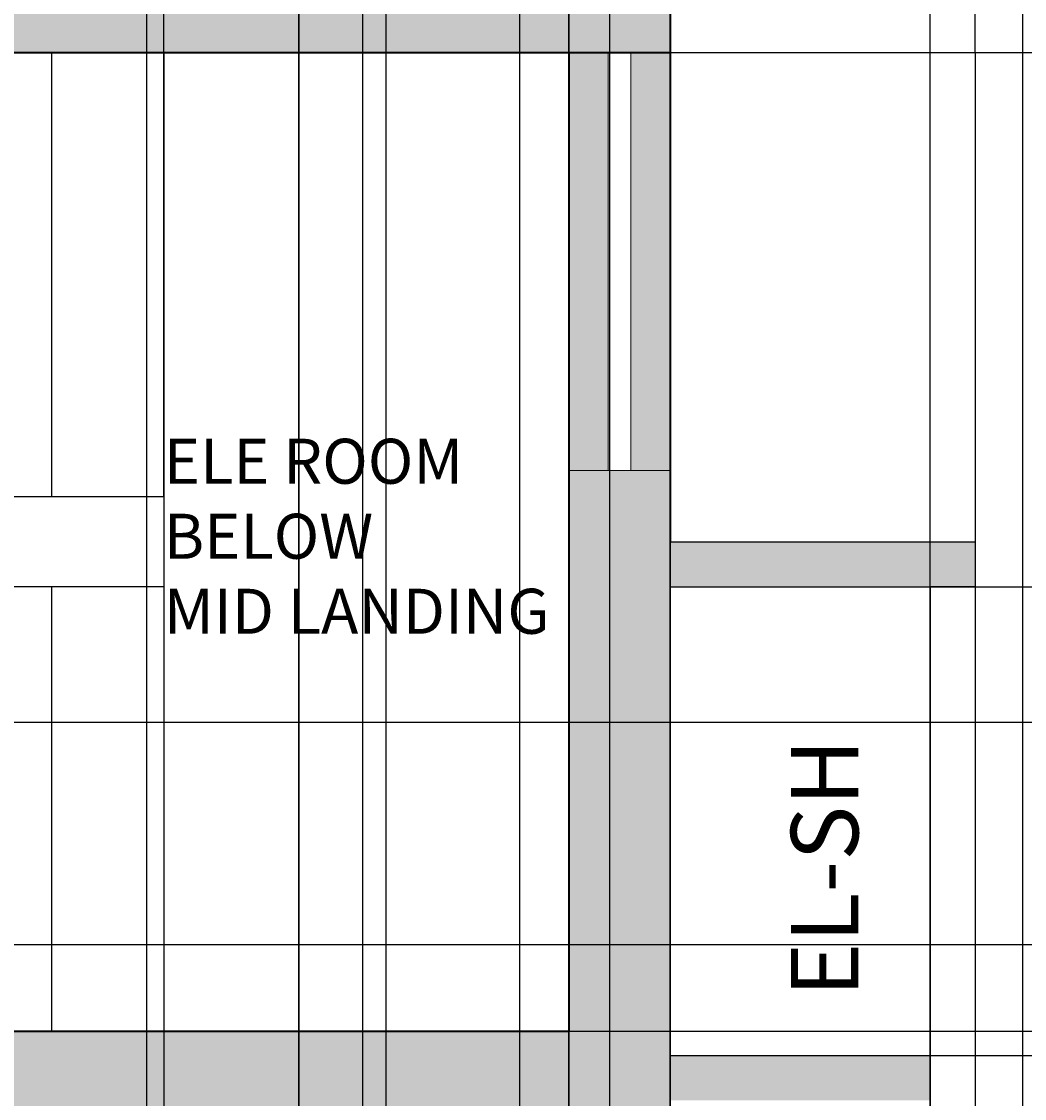
# Model space of a CAD drawing. Units: inches. Extents: x 818 to 1898, y 976 to 2364.
# Tile 49 of 96: x 1657 to 1746, y 1594 to 1690. Entities that reach past the tile are written whole.
import ezdxf

# ---------------------------------------------------------------- set-up
doc = ezdxf.new("R2010")
doc.units = ezdxf.units.IN
doc.header["$LTSCALE"] = 5
doc.header["$MEASUREMENT"] = 0
for name, color, linetype, lineweight in [('A-ANNO-DIMS', 2, 'Continuous', 18), ('A-ANNO-TEXT', 7, 'Continuous', 18), ('A-AREA-IDEN', 7, 'Continuous', 18), ('A-FLOR-SHFT', 7, 'Continuous', 25), ('A-FLOR-STRS', 7, 'Continuous', 25), ('A-GLAZ', 4, 'Continuous', 18), ('A-WALL', 7, 'Continuous', 40)]:
    doc.layers.add(name, color=color, linetype=linetype, lineweight=lineweight)
doc.layers.add('A-GLAZ-PATT', color=141, linetype='Continuous', lineweight=9, true_color=0xadddf7)
doc.layers.add('A-WALL-PATT', color=251, linetype='Continuous', lineweight=13, true_color=0x636466)
doc.styles.get("Standard").update_dxf_attribs({"font": 'arial.ttf'})
doc.dimstyles.get("Standard").update_dxf_attribs({"dimtxt": 0.18, "dimasz": 0.18, "dimexe": 0.18, "dimexo": 0.0625, "dimgap": 0.09, "dimtad": 0, "dimtih": 1, "dimtoh": 1, "dimdec": 4, "dimzin": 0, "dimdsep": 46, "dimtxsty": 'Standard', "dimcen": 0.09, "dimadec": 0, "dimazin": 0, "dimtfac": 1, "dimtdec": 4, "dimtofl": 0, "dimtmove": 0, "dimatfit": 3, "dimfxl": 1, "dimtolj": 1, "dimtzin": 0, "dimarcsym": 0})

# ---------------------------------------------------------------- blocks, each defined once
blk = doc.blocks.new('*D71')
at = {"layer": 'A-ANNO-DIMS', "color": 0, "lineweight": -2, "ltscale": 5, "transparency": 16777216}
for p, q in [((1714.788, 2053.078), (1897.916, 2053.078)), ((1897.736, 2052.898), (1897.736, 1699.76)), ((1897.736, 1346.258), (1897.736, 1699.396)), ((1714.788, 1346.078), (1897.916, 1346.078))]:
    blk.add_line(p, q, dxfattribs=at)
at = {"layer": 'A-ANNO-DIMS', "color": 0, "ltscale": 5, "transparency": 16777216}
for points in [[(1897.706, 2052.898), (1897.766, 2052.898), (1897.736, 2053.078)], [(1897.706, 1346.258), (1897.766, 1346.258), (1897.736, 1346.078)]]:
    blk.add_solid(points, dxfattribs=at)
at = {"layer": 'Defpoints', "color": 0, "ltscale": 5, "transparency": 16777216}
for p in [(1714.725, 2053.078), (1897.736, 2053.078), (1714.725, 1346.078)]:
    blk.add_point(p, dxfattribs=at)
at = {"layer": 'A-ANNO-DIMS', "color": 0, "ltscale": 5, "transparency": 16777216, "insert": (1897.736, 1699.578), "char_height": 0.18, "attachment_point": 5}
blk.add_mtext('\\A1;707', dxfattribs=at)
blk = doc.blocks.new('*D103')
at = {"layer": 'A-ANNO-DIMS', "color": 0, "lineweight": -2, "ltscale": 5, "transparency": 16777216}
for p, q in [((1626.575, 1071.118), (1626.575, 2363.873)), ((1626.755, 2363.693), (1657.699, 2363.693)), ((1689.291, 2363.693), (1658.348, 2363.693)), ((1689.471, 1071.118), (1689.471, 2363.873))]:
    blk.add_line(p, q, dxfattribs=at)
at = {"layer": 'A-ANNO-DIMS', "color": 0, "ltscale": 5, "transparency": 16777216}
for points in [[(1626.755, 2363.723), (1626.755, 2363.663), (1626.575, 2363.693)], [(1689.291, 2363.723), (1689.291, 2363.663), (1689.471, 2363.693)]]:
    blk.add_solid(points, dxfattribs=at)
at = {"layer": 'Defpoints', "color": 0, "ltscale": 5, "transparency": 16777216}
for p in [(1689.471, 2363.693), (1626.575, 1071.055), (1689.471, 1071.055)]:
    blk.add_point(p, dxfattribs=at)
at = {"layer": 'A-ANNO-DIMS', "color": 0, "ltscale": 5, "transparency": 16777216, "insert": (1658.023, 2363.693), "char_height": 0.18, "attachment_point": 5}
blk.add_mtext('\\A1;62.9', dxfattribs=at)
blk = doc.blocks.new('*D104')
at = {"layer": 'A-ANNO-DIMS', "color": 0, "lineweight": -2, "ltscale": 5, "transparency": 16777216}
for p, q in [((1689.471, 1071.118), (1689.471, 2363.873)), ((1689.651, 2363.693), (1717.401, 2363.693)), ((1745.903, 2363.693), (1718.154, 2363.693)), ((1746.083, 1071.118), (1746.083, 2363.873))]:
    blk.add_line(p, q, dxfattribs=at)
at = {"layer": 'A-ANNO-DIMS', "color": 0, "ltscale": 5, "transparency": 16777216}
for points in [[(1689.651, 2363.723), (1689.651, 2363.663), (1689.471, 2363.693)], [(1745.903, 2363.723), (1745.903, 2363.663), (1746.083, 2363.693)]]:
    blk.add_solid(points, dxfattribs=at)
at = {"layer": 'Defpoints', "color": 0, "ltscale": 5, "transparency": 16777216}
for p in [(1746.083, 2363.693), (1689.471, 1071.055), (1746.083, 1071.055)]:
    blk.add_point(p, dxfattribs=at)
at = {"layer": 'A-ANNO-DIMS', "color": 0, "ltscale": 5, "transparency": 16777216, "insert": (1717.777, 2363.693), "char_height": 0.18, "attachment_point": 5}
blk.add_mtext('\\A1;56.61', dxfattribs=at)
blk = doc.blocks.new('*D118')
at = {"layer": 'A-ANNO-DIMS', "color": 0, "lineweight": -2, "ltscale": 5, "transparency": 16777216}
for p, q in [((1766.29, 1627.505), (818.026, 1627.505)), ((818.206, 1627.325), (818.206, 1586.526)), ((818.206, 1545.363), (818.206, 1586.162)), ((1766.29, 1545.183), (818.026, 1545.183))]:
    blk.add_line(p, q, dxfattribs=at)
at = {"layer": 'A-ANNO-DIMS', "color": 0, "ltscale": 5, "transparency": 16777216}
for points in [[(818.176, 1627.325), (818.236, 1627.325), (818.206, 1627.505)], [(818.176, 1545.363), (818.236, 1545.363), (818.206, 1545.183)]]:
    blk.add_solid(points, dxfattribs=at)
at = {"layer": 'Defpoints', "color": 0, "ltscale": 5, "transparency": 16777216}
for p in [(818.206, 1627.505), (1766.352, 1627.505), (1766.352, 1545.183)]:
    blk.add_point(p, dxfattribs=at)
at = {"layer": 'A-ANNO-DIMS', "color": 0, "ltscale": 5, "transparency": 16777216, "insert": (818.206, 1586.344), "char_height": 0.18, "attachment_point": 5}
blk.add_mtext('\\A1;82.32', dxfattribs=at)
blk = doc.blocks.new('*D119')
at = {"layer": 'A-ANNO-DIMS', "color": 0, "lineweight": -2, "ltscale": 5, "transparency": 16777216}
for p, q in [((1766.29, 1716.987), (818.026, 1716.987)), ((818.206, 1716.807), (818.206, 1672.428)), ((818.206, 1627.685), (818.206, 1672.064)), ((1766.29, 1627.505), (818.026, 1627.505))]:
    blk.add_line(p, q, dxfattribs=at)
at = {"layer": 'A-ANNO-DIMS', "color": 0, "ltscale": 5, "transparency": 16777216}
for points in [[(818.176, 1716.807), (818.236, 1716.807), (818.206, 1716.987)], [(818.176, 1627.685), (818.236, 1627.685), (818.206, 1627.505)]]:
    blk.add_solid(points, dxfattribs=at)
at = {"layer": 'Defpoints', "color": 0, "ltscale": 5, "transparency": 16777216}
for p in [(818.206, 1716.987), (1766.352, 1716.987), (1766.352, 1627.505)]:
    blk.add_point(p, dxfattribs=at)
at = {"layer": 'A-ANNO-DIMS', "color": 0, "ltscale": 5, "transparency": 16777216, "insert": (818.206, 1672.246), "char_height": 0.18, "attachment_point": 5}
blk.add_mtext('\\A1;89.48', dxfattribs=at)
blk = doc.blocks.new('*D154')
at = {"layer": 'A-ANNO-DIMS', "color": 0, "lineweight": -2, "ltscale": 5, "transparency": 16777216}
for p, q in [((1701.369, 1290.141), (1701.369, 2363.873)), ((1701.549, 2363.693), (1705.22, 2363.693)), ((1709.189, 2363.693), (1705.518, 2363.693)), ((1709.369, 1298.141), (1709.369, 2363.873))]:
    blk.add_line(p, q, dxfattribs=at)
at = {"layer": 'A-ANNO-DIMS', "color": 0, "ltscale": 5, "transparency": 16777216}
for points in [[(1701.549, 2363.723), (1701.549, 2363.663), (1701.369, 2363.693)], [(1709.189, 2363.723), (1709.189, 2363.663), (1709.369, 2363.693)]]:
    blk.add_solid(points, dxfattribs=at)
at = {"layer": 'Defpoints', "color": 0, "ltscale": 5, "transparency": 16777216}
for p in [(1709.369, 2363.693), (1709.369, 1298.078), (1701.369, 1290.078)]:
    blk.add_point(p, dxfattribs=at)
at = {"layer": 'A-ANNO-DIMS', "color": 0, "ltscale": 5, "transparency": 16777216, "insert": (1705.369, 2363.693), "char_height": 0.18, "attachment_point": 5}
blk.add_mtext('\\A1;8', dxfattribs=at)
blk = doc.blocks.new('*D170')
at = {"layer": 'A-ANNO-DIMS', "color": 0, "lineweight": -2, "ltscale": 5, "transparency": 16777216}
for p, q in [((1430.788, 1600.078), (1897.916, 1600.078)), ((1897.736, 1599.898), (1897.736, 1550.76)), ((1897.736, 1501.258), (1897.736, 1550.396)), ((1430.788, 1501.078), (1897.916, 1501.078))]:
    blk.add_line(p, q, dxfattribs=at)
at = {"layer": 'A-ANNO-DIMS', "color": 0, "ltscale": 5, "transparency": 16777216}
for points in [[(1897.706, 1599.898), (1897.766, 1599.898), (1897.736, 1600.078)], [(1897.706, 1501.258), (1897.766, 1501.258), (1897.736, 1501.078)]]:
    blk.add_solid(points, dxfattribs=at)
at = {"layer": 'Defpoints', "color": 0, "ltscale": 5, "transparency": 16777216}
for p in [(1430.725, 1600.078), (1897.736, 1600.078), (1430.725, 1501.078)]:
    blk.add_point(p, dxfattribs=at)
at = {"layer": 'A-ANNO-DIMS', "color": 0, "ltscale": 5, "transparency": 16777216, "insert": (1897.736, 1550.578), "char_height": 0.18, "attachment_point": 5}
blk.add_mtext('\\A1;99', dxfattribs=at)
blk = doc.blocks.new('*D175')
at = {"layer": 'A-ANNO-DIMS', "color": 0, "lineweight": -2, "ltscale": 5, "transparency": 16777216}
for p, q in [((1559.725, 1647.641), (1559.725, 2363.873)), ((1559.905, 2363.693), (1614.445, 2363.693)), ((1669.545, 2363.693), (1615.005, 2363.693)), ((1669.725, 1647.641), (1669.725, 2363.873))]:
    blk.add_line(p, q, dxfattribs=at)
at = {"layer": 'A-ANNO-DIMS', "color": 0, "ltscale": 5, "transparency": 16777216}
for points in [[(1559.905, 2363.723), (1559.905, 2363.663), (1559.725, 2363.693)], [(1669.545, 2363.723), (1669.545, 2363.663), (1669.725, 2363.693)]]:
    blk.add_solid(points, dxfattribs=at)
at = {"layer": 'Defpoints', "color": 0, "ltscale": 5, "transparency": 16777216}
for p in [(1669.725, 2363.693), (1559.725, 1647.578), (1669.725, 1647.578)]:
    blk.add_point(p, dxfattribs=at)
at = {"layer": 'A-ANNO-DIMS', "color": 0, "ltscale": 5, "transparency": 16777216, "insert": (1614.725, 2363.693), "char_height": 0.18, "attachment_point": 5}
blk.add_mtext('\\A1;110', dxfattribs=at)
blk = doc.blocks.new('*D178')
at = {"layer": 'A-ANNO-DIMS', "color": 0, "lineweight": -2, "ltscale": 5, "transparency": 16777216}
for p, q in [((1669.725, 1600.016), (1669.725, 975.663)), ((1705.725, 1600.016), (1705.725, 975.663)), ((1669.905, 975.843), (1687.506, 975.843)), ((1705.545, 975.843), (1687.944, 975.843))]:
    blk.add_line(p, q, dxfattribs=at)
at = {"layer": 'A-ANNO-DIMS', "color": 0, "ltscale": 5, "transparency": 16777216}
for points in [[(1669.905, 975.873), (1669.905, 975.813), (1669.725, 975.843)], [(1705.545, 975.873), (1705.545, 975.813), (1705.725, 975.843)]]:
    blk.add_solid(points, dxfattribs=at)
at = {"layer": 'Defpoints', "color": 0, "ltscale": 5, "transparency": 16777216}
for p in [(1669.725, 1600.078), (1705.725, 1600.078), (1705.725, 975.843)]:
    blk.add_point(p, dxfattribs=at)
at = {"layer": 'A-ANNO-DIMS', "color": 0, "ltscale": 5, "transparency": 16777216, "insert": (1687.725, 975.843), "char_height": 0.18, "attachment_point": 5}
blk.add_mtext('\\A1;36', dxfattribs=at)
blk = doc.blocks.new('*D179')
at = {"layer": 'A-ANNO-DIMS', "color": 0, "lineweight": -2, "ltscale": 5, "transparency": 16777216}
for p, q in [((1669.788, 1687.078), (1897.916, 1687.078)), ((1897.736, 1686.898), (1897.736, 1643.76)), ((1897.736, 1600.258), (1897.736, 1643.396)), ((1669.788, 1600.078), (1897.916, 1600.078))]:
    blk.add_line(p, q, dxfattribs=at)
at = {"layer": 'A-ANNO-DIMS', "color": 0, "ltscale": 5, "transparency": 16777216}
for points in [[(1897.706, 1686.898), (1897.766, 1686.898), (1897.736, 1687.078)], [(1897.706, 1600.258), (1897.766, 1600.258), (1897.736, 1600.078)]]:
    blk.add_solid(points, dxfattribs=at)
at = {"layer": 'Defpoints', "color": 0, "ltscale": 5, "transparency": 16777216}
for p in [(1669.725, 1687.078), (1897.736, 1687.078), (1669.725, 1600.078)]:
    blk.add_point(p, dxfattribs=at)
at = {"layer": 'A-ANNO-DIMS', "color": 0, "ltscale": 5, "transparency": 16777216, "insert": (1897.736, 1643.578), "char_height": 0.18, "attachment_point": 5}
blk.add_mtext('\\A1;87', dxfattribs=at)
blk = doc.blocks.new('*D180')
at = {"layer": 'A-ANNO-DIMS', "color": 0, "lineweight": -2, "ltscale": 5, "transparency": 16777216}
for p, q in [((1599.725, 1639.516), (1599.725, 975.663)), ((1669.725, 1639.516), (1669.725, 975.663)), ((1599.905, 975.843), (1634.507, 975.843)), ((1669.545, 975.843), (1634.943, 975.843))]:
    blk.add_line(p, q, dxfattribs=at)
at = {"layer": 'A-ANNO-DIMS', "color": 0, "ltscale": 5, "transparency": 16777216}
for points in [[(1599.905, 975.873), (1599.905, 975.813), (1599.725, 975.843)], [(1669.545, 975.873), (1669.545, 975.813), (1669.725, 975.843)]]:
    blk.add_solid(points, dxfattribs=at)
at = {"layer": 'Defpoints', "color": 0, "ltscale": 5, "transparency": 16777216}
for p in [(1599.725, 1639.578), (1669.725, 1639.578), (1669.725, 975.843)]:
    blk.add_point(p, dxfattribs=at)
at = {"layer": 'A-ANNO-DIMS', "color": 0, "ltscale": 5, "transparency": 16777216, "insert": (1634.725, 975.843), "char_height": 0.18, "attachment_point": 5}
blk.add_mtext('\\A1;70', dxfattribs=at)
blk = doc.blocks.new('*D185')
at = {"layer": 'A-ANNO-DIMS', "color": 0, "lineweight": -2, "ltscale": 5, "transparency": 16777216}
for p, q in [((1737.903, 1639.578), (1897.916, 1639.578)), ((1897.736, 1639.398), (1897.736, 1618.93)), ((1897.736, 1598.098), (1897.736, 1618.566)), ((1737.903, 1597.918), (1897.916, 1597.918))]:
    blk.add_line(p, q, dxfattribs=at)
at = {"layer": 'A-ANNO-DIMS', "color": 0, "ltscale": 5, "transparency": 16777216}
for points in [[(1897.706, 1639.398), (1897.766, 1639.398), (1897.736, 1639.578)], [(1897.706, 1598.098), (1897.766, 1598.098), (1897.736, 1597.918)]]:
    blk.add_solid(points, dxfattribs=at)
at = {"layer": 'Defpoints', "color": 0, "ltscale": 5, "transparency": 16777216}
for p in [(1737.841, 1639.578), (1897.736, 1639.578), (1737.841, 1597.918)]:
    blk.add_point(p, dxfattribs=at)
at = {"layer": 'A-ANNO-DIMS', "color": 0, "ltscale": 5, "transparency": 16777216, "insert": (1897.736, 1618.748), "char_height": 0.18, "attachment_point": 5}
blk.add_mtext('\\A1;41.66', dxfattribs=at)
blk = doc.blocks.new('*D186')
at = {"layer": 'A-ANNO-DIMS', "color": 0, "lineweight": -2, "ltscale": 5, "transparency": 16777216}
for p, q in [((1714.725, 1549.141), (1714.725, 2363.873)), ((1714.905, 2363.693), (1725.818, 2363.693)), ((1737.661, 2363.693), (1726.748, 2363.693)), ((1737.841, 1549.141), (1737.841, 2363.873))]:
    blk.add_line(p, q, dxfattribs=at)
at = {"layer": 'A-ANNO-DIMS', "color": 0, "ltscale": 5, "transparency": 16777216}
for points in [[(1714.905, 2363.723), (1714.905, 2363.663), (1714.725, 2363.693)], [(1737.661, 2363.723), (1737.661, 2363.663), (1737.841, 2363.693)]]:
    blk.add_solid(points, dxfattribs=at)
at = {"layer": 'Defpoints', "color": 0, "ltscale": 5, "transparency": 16777216}
for p in [(1737.841, 2363.693), (1714.725, 1549.078), (1737.841, 1549.078)]:
    blk.add_point(p, dxfattribs=at)
at = {"layer": 'A-ANNO-DIMS', "color": 0, "ltscale": 5, "transparency": 16777216, "insert": (1726.283, 2363.693), "char_height": 0.18, "attachment_point": 5}
blk.add_mtext('\\A1;23.116', dxfattribs=at)
blk = doc.blocks.new('*D195')
at = {"layer": 'A-ANNO-DIMS', "color": 0, "lineweight": -2, "ltscale": 5, "transparency": 16777216}
for p, q in [((1681.725, 1379.141), (1681.725, 2363.873)), ((1681.905, 2363.693), (1693.505, 2363.693)), ((1705.545, 2363.693), (1693.945, 2363.693)), ((1705.725, 1355.141), (1705.725, 2363.873))]:
    blk.add_line(p, q, dxfattribs=at)
at = {"layer": 'A-ANNO-DIMS', "color": 0, "ltscale": 5, "transparency": 16777216}
for points in [[(1681.905, 2363.723), (1681.905, 2363.663), (1681.725, 2363.693)], [(1705.545, 2363.723), (1705.545, 2363.663), (1705.725, 2363.693)]]:
    blk.add_solid(points, dxfattribs=at)
at = {"layer": 'Defpoints', "color": 0, "ltscale": 5, "transparency": 16777216}
for p in [(1705.725, 2363.693), (1681.725, 1379.078), (1705.725, 1355.078)]:
    blk.add_point(p, dxfattribs=at)
at = {"layer": 'A-ANNO-DIMS', "color": 0, "ltscale": 5, "transparency": 16777216, "insert": (1693.725, 2363.693), "char_height": 0.18, "attachment_point": 5}
blk.add_mtext('\\A1;24', dxfattribs=at)
blk = doc.blocks.new('*D199')
at = {"layer": 'A-ANNO-DIMS', "color": 0, "lineweight": -2, "ltscale": 5, "transparency": 16777216}
for p, q in [((1559.788, 1687.078), (1897.916, 1687.078)), ((1897.736, 1686.898), (1897.736, 1513.154)), ((1897.736, 1339.045), (1897.736, 1512.79)), ((1660.377, 1338.865), (1897.916, 1338.865))]:
    blk.add_line(p, q, dxfattribs=at)
at = {"layer": 'A-ANNO-DIMS', "color": 0, "ltscale": 5, "transparency": 16777216}
for points in [[(1897.706, 1686.898), (1897.766, 1686.898), (1897.736, 1687.078)], [(1897.706, 1339.045), (1897.766, 1339.045), (1897.736, 1338.865)]]:
    blk.add_solid(points, dxfattribs=at)
at = {"layer": 'Defpoints', "color": 0, "ltscale": 5, "transparency": 16777216}
for p in [(1559.725, 1687.078), (1897.736, 1687.078), (1660.314, 1338.865)]:
    blk.add_point(p, dxfattribs=at)
at = {"layer": 'A-ANNO-DIMS', "color": 0, "ltscale": 5, "transparency": 16777216, "insert": (1897.736, 1512.972), "char_height": 0.18, "attachment_point": 5}
blk.add_mtext('\\A1;348.2', dxfattribs=at)
blk = doc.blocks.new('*D212')
at = {"layer": 'A-ANNO-DIMS', "color": 0, "lineweight": -2, "ltscale": 5, "transparency": 16777216}
for p, q in [((1681.725, 1900.016), (1681.725, 975.663)), ((1705.725, 1876.016), (1705.725, 975.663)), ((1681.905, 975.843), (1693.505, 975.843)), ((1705.545, 975.843), (1693.945, 975.843))]:
    blk.add_line(p, q, dxfattribs=at)
at = {"layer": 'A-ANNO-DIMS', "color": 0, "ltscale": 5, "transparency": 16777216}
for points in [[(1681.905, 975.873), (1681.905, 975.813), (1681.725, 975.843)], [(1705.545, 975.873), (1705.545, 975.813), (1705.725, 975.843)]]:
    blk.add_solid(points, dxfattribs=at)
at = {"layer": 'Defpoints', "color": 0, "ltscale": 5, "transparency": 16777216}
for p in [(1681.725, 1900.078), (1705.725, 1876.078), (1705.725, 975.843)]:
    blk.add_point(p, dxfattribs=at)
at = {"layer": 'A-ANNO-DIMS', "color": 0, "ltscale": 5, "transparency": 16777216, "insert": (1693.725, 975.843), "char_height": 0.18, "attachment_point": 5}
blk.add_mtext('\\A1;24', dxfattribs=at)
blk = doc.blocks.new('*D214')
at = {"layer": 'A-ANNO-DIMS', "color": 0, "lineweight": -2, "ltscale": 5, "transparency": 16777216}
for p, q in [((1511.725, 1687.016), (1511.725, 975.663)), ((1714.725, 1687.016), (1714.725, 975.663)), ((1511.905, 975.843), (1612.935, 975.843)), ((1714.545, 975.843), (1613.516, 975.843))]:
    blk.add_line(p, q, dxfattribs=at)
at = {"layer": 'A-ANNO-DIMS', "color": 0, "ltscale": 5, "transparency": 16777216}
for points in [[(1511.905, 975.873), (1511.905, 975.813), (1511.725, 975.843)], [(1714.545, 975.873), (1714.545, 975.813), (1714.725, 975.843)]]:
    blk.add_solid(points, dxfattribs=at)
at = {"layer": 'Defpoints', "color": 0, "ltscale": 5, "transparency": 16777216}
for p in [(1511.725, 1687.078), (1714.725, 1687.078), (1714.725, 975.843)]:
    blk.add_point(p, dxfattribs=at)
at = {"layer": 'A-ANNO-DIMS', "color": 0, "ltscale": 5, "transparency": 16777216, "insert": (1613.225, 975.843), "char_height": 0.18, "attachment_point": 5}
blk.add_mtext('\\A1;203', dxfattribs=at)
blk = doc.blocks.new('*D221')
at = {"layer": 'A-ANNO-DIMS', "color": 0, "lineweight": -2, "ltscale": 5, "transparency": 16777216}
for p, q in [((1668.184, 1696.016), (1668.184, 975.663)), ((1705.725, 1696.016), (1705.725, 975.663)), ((1668.364, 975.843), (1686.561, 975.843)), ((1705.545, 975.843), (1687.348, 975.843))]:
    blk.add_line(p, q, dxfattribs=at)
at = {"layer": 'A-ANNO-DIMS', "color": 0, "ltscale": 5, "transparency": 16777216}
for points in [[(1668.364, 975.873), (1668.364, 975.813), (1668.184, 975.843)], [(1705.545, 975.873), (1705.545, 975.813), (1705.725, 975.843)]]:
    blk.add_solid(points, dxfattribs=at)
at = {"layer": 'Defpoints', "color": 0, "ltscale": 5, "transparency": 16777216}
for p in [(1668.184, 1696.078), (1705.725, 1696.078), (1705.725, 975.843)]:
    blk.add_point(p, dxfattribs=at)
at = {"layer": 'A-ANNO-DIMS', "color": 0, "ltscale": 5, "transparency": 16777216, "insert": (1686.955, 975.843), "char_height": 0.18, "attachment_point": 5}
blk.add_mtext('\\A1;37.54', dxfattribs=at)
blk = doc.blocks.new('*D228')
at = {"layer": 'A-ANNO-DIMS', "color": 0, "lineweight": -2, "ltscale": 5, "transparency": 16777216}
for p, q in [((1687.394, 1802.016), (1687.394, 975.663)), ((1705.725, 1802.016), (1705.725, 975.663)), ((1687.574, 975.843), (1696.174, 975.843)), ((1705.545, 975.843), (1696.945, 975.843))]:
    blk.add_line(p, q, dxfattribs=at)
at = {"layer": 'A-ANNO-DIMS', "color": 0, "ltscale": 5, "transparency": 16777216}
for points in [[(1687.574, 975.873), (1687.574, 975.813), (1687.394, 975.843)], [(1705.545, 975.873), (1705.545, 975.813), (1705.725, 975.843)]]:
    blk.add_solid(points, dxfattribs=at)
at = {"layer": 'Defpoints', "color": 0, "ltscale": 5, "transparency": 16777216}
for p in [(1687.394, 1802.078), (1705.725, 1802.078), (1705.725, 975.843)]:
    blk.add_point(p, dxfattribs=at)
at = {"layer": 'A-ANNO-DIMS', "color": 0, "ltscale": 5, "transparency": 16777216, "insert": (1696.56, 975.843), "char_height": 0.18, "attachment_point": 5}
blk.add_mtext('\\A1;18.33', dxfattribs=at)
blk = doc.blocks.new('*D267')
at = {"layer": 'A-ANNO-DIMS', "color": 0, "lineweight": -2, "ltscale": 5, "transparency": 16777216}
for p, q in [((1714.725, 1687.016), (1714.725, 975.663)), ((1741.841, 1687.016), (1741.841, 975.663)), ((1714.905, 975.843), (1727.818, 975.843)), ((1741.661, 975.843), (1728.748, 975.843))]:
    blk.add_line(p, q, dxfattribs=at)
at = {"layer": 'A-ANNO-DIMS', "color": 0, "ltscale": 5, "transparency": 16777216}
for points in [[(1714.905, 975.873), (1714.905, 975.813), (1714.725, 975.843)], [(1741.661, 975.873), (1741.661, 975.813), (1741.841, 975.843)]]:
    blk.add_solid(points, dxfattribs=at)
at = {"layer": 'Defpoints', "color": 0, "ltscale": 5, "transparency": 16777216}
for p in [(1714.725, 1687.078), (1741.841, 1687.078), (1741.841, 975.843)]:
    blk.add_point(p, dxfattribs=at)
at = {"layer": 'A-ANNO-DIMS', "color": 0, "ltscale": 5, "transparency": 16777216, "insert": (1728.283, 975.843), "char_height": 0.18, "attachment_point": 5}
blk.add_mtext('\\A1;27.116', dxfattribs=at)
blk = doc.blocks.new('*D268')
at = {"layer": 'A-ANNO-DIMS', "color": 0, "lineweight": -2, "ltscale": 5, "transparency": 16777216}
for p, q in [((1741.903, 1890.29), (1897.916, 1890.29)), ((1897.736, 1890.11), (1897.736, 1788.866)), ((1897.736, 1687.258), (1897.736, 1788.502)), ((1741.903, 1687.078), (1897.916, 1687.078))]:
    blk.add_line(p, q, dxfattribs=at)
at = {"layer": 'A-ANNO-DIMS', "color": 0, "ltscale": 5, "transparency": 16777216}
for points in [[(1897.706, 1890.11), (1897.766, 1890.11), (1897.736, 1890.29)], [(1897.706, 1687.258), (1897.766, 1687.258), (1897.736, 1687.078)]]:
    blk.add_solid(points, dxfattribs=at)
at = {"layer": 'Defpoints', "color": 0, "ltscale": 5, "transparency": 16777216}
for p in [(1741.841, 1890.29), (1897.736, 1890.29), (1741.841, 1687.078)]:
    blk.add_point(p, dxfattribs=at)
at = {"layer": 'A-ANNO-DIMS', "color": 0, "ltscale": 5, "transparency": 16777216, "insert": (1897.736, 1788.684), "char_height": 0.18, "attachment_point": 5}
blk.add_mtext('\\A1;203.2', dxfattribs=at)
blk = doc.blocks.new('*D282')
at = {"layer": 'A-ANNO-DIMS', "color": 0, "lineweight": -2, "ltscale": 5, "transparency": 16777216}
for p, q in [((1422.083, 2081.188), (1897.916, 2081.188)), ((1897.736, 2081.008), (1897.736, 1884.315)), ((1897.736, 1687.258), (1897.736, 1883.951)), ((1463.788, 1687.078), (1897.916, 1687.078))]:
    blk.add_line(p, q, dxfattribs=at)
at = {"layer": 'A-ANNO-DIMS', "color": 0, "ltscale": 5, "transparency": 16777216}
for points in [[(1897.706, 2081.008), (1897.766, 2081.008), (1897.736, 2081.188)], [(1897.706, 1687.258), (1897.766, 1687.258), (1897.736, 1687.078)]]:
    blk.add_solid(points, dxfattribs=at)
at = {"layer": 'Defpoints', "color": 0, "ltscale": 5, "transparency": 16777216}
for p in [(1422.02, 2081.188), (1897.736, 2081.188), (1463.725, 1687.078)]:
    blk.add_point(p, dxfattribs=at)
at = {"layer": 'A-ANNO-DIMS', "color": 0, "ltscale": 5, "transparency": 16777216, "insert": (1897.736, 1884.133), "char_height": 0.18, "attachment_point": 5}
blk.add_mtext('\\A1;394.1', dxfattribs=at)
blk = doc.blocks.new('*D291')
at = {"layer": 'A-ANNO-DIMS', "color": 0, "lineweight": -2, "ltscale": 5, "transparency": 16777216}
for p, q in [((1206.788, 1687.078), (1897.916, 1687.078)), ((1897.736, 1686.898), (1897.736, 1647.606)), ((1897.736, 1607.951), (1897.736, 1647.242)), ((1318.956, 1607.771), (1897.916, 1607.771))]:
    blk.add_line(p, q, dxfattribs=at)
at = {"layer": 'A-ANNO-DIMS', "color": 0, "ltscale": 5, "transparency": 16777216}
for points in [[(1897.706, 1686.898), (1897.766, 1686.898), (1897.736, 1687.078)], [(1897.706, 1607.951), (1897.766, 1607.951), (1897.736, 1607.771)]]:
    blk.add_solid(points, dxfattribs=at)
at = {"layer": 'Defpoints', "color": 0, "ltscale": 5, "transparency": 16777216}
for p in [(1206.725, 1687.078), (1897.736, 1687.078), (1318.893, 1607.771)]:
    blk.add_point(p, dxfattribs=at)
at = {"layer": 'A-ANNO-DIMS', "color": 0, "ltscale": 5, "transparency": 16777216, "insert": (1897.736, 1647.424), "char_height": 0.18, "attachment_point": 5}
blk.add_mtext('\\A1;79.3', dxfattribs=at)

msp = doc.modelspace()

# ---------------------------------------------------------------- hatches: boundary and pattern name
at = {"layer": 'A-GLAZ-PATT', "ltscale": 5}
h = msp.add_hatch(color=256, dxfattribs=at)
h.dxf.hatch_style = 1
h.paths.add_polyline_path([(1283.8183, 1504.5782), (1206.7251, 1504.5782), (1206.7251, 1501.0782), (1283.8183, 1501.0782)])
h.paths.add_polyline_path([(1283.8183, 1510.0782), (1206.7251, 1510.0782), (1206.7251, 1506.5782), (1283.8183, 1506.5782)])
h.paths.add_polyline_path([(1490.9163, 1355.0782), (1439.7252, 1355.0782), (1439.7252, 1409.0522), (1436.2252, 1409.0522), (1436.2252, 1351.5782), (1490.9163, 1351.5782)])
h.paths.add_polyline_path([(1434.2252, 1409.0522), (1430.7251, 1409.0522), (1430.7251, 1346.0782), (1435.0799, 1346.0782), (1435.0731, 1346.1152), (1435.1501, 1346.0782), (1490.9163, 1346.0782), (1490.9163, 1349.5782), (1434.2252, 1349.5782)])
h.paths.add_polyline_path([(1714.7251, 1545.0782), (1711.2252, 1545.0782), (1711.2252, 1521.0782), (1714.7251, 1521.0782)])
h.paths.add_polyline_path([(1709.2252, 1545.0782), (1705.7251, 1545.0782), (1705.7251, 1521.0782), (1709.2252, 1521.0782)])
h.paths.add_polyline_path([(1714.7251, 1687.0782), (1711.2252, 1687.0782), (1711.2252, 1649.9029), (1714.7251, 1649.9029)])
h.paths.add_polyline_path([(1709.2252, 1687.0782), (1705.7251, 1687.0782), (1705.7251, 1649.9029), (1709.2252, 1649.9029)])
h.paths.add_polyline_path([(1709.2252, 1745.5584), (1705.7251, 1745.5584), (1705.7251, 1717.3178), (1709.2252, 1717.3178)])
h.paths.add_polyline_path([(1714.7251, 1745.5584), (1711.2252, 1745.5584), (1711.2252, 1717.3178), (1714.7251, 1717.3178)])
h.paths.add_polyline_path([(1714.7251, 2014.5114), (1711.2252, 2014.5114), (1711.2252, 1962.0338), (1714.7251, 1962.0338)])
h.paths.add_polyline_path([(1709.2252, 2014.5114), (1705.7251, 2014.5114), (1705.7251, 1962.0338), (1709.2252, 1962.0338)])
h.paths.add_polyline_path([(1538.5155, 2047.5782), (1485.1216, 2047.5782), (1485.1216, 2044.0782), (1538.5155, 2044.0782)])
h.paths.add_polyline_path([(1538.5155, 2053.0782), (1485.1216, 2053.0782), (1485.1216, 2049.5782), (1538.5155, 2049.5782)])
h.paths.add_polyline_path([(1388.0315, 2047.5782), (1330.305, 2047.5782), (1330.305, 2044.0782), (1388.0315, 2044.0782)])
h.paths.add_polyline_path([(1388.0315, 2053.0782), (1330.305, 2053.0782), (1330.305, 2049.5782), (1388.0315, 2049.5782)])
h.paths.add_polyline_path([(1262.2252, 2019.2871), (1258.7252, 2019.2871), (1258.7252, 1928.9218), (1262.2252, 1928.9218)])
h.paths.add_polyline_path([(1267.7252, 2019.2871), (1264.2252, 2019.2871), (1264.2252, 1928.9218), (1267.7252, 1928.9218)])
h.paths.add_polyline_path([(1262.2252, 1862.9652), (1258.7252, 1862.9652), (1258.7252, 1814.9652), (1262.2252, 1814.9652)])
h.paths.add_polyline_path([(1267.7252, 1862.9652), (1264.2252, 1862.9652), (1264.2252, 1814.9652), (1267.7252, 1814.9652)])
h.paths.add_polyline_path([(1262.2252, 1755.3321), (1258.7252, 1755.3321), (1258.7252, 1707.3321), (1262.2252, 1707.3321)])
h.paths.add_polyline_path([(1267.7252, 1755.3321), (1264.2252, 1755.3321), (1264.2252, 1707.3321), (1267.7252, 1707.3321)])
h.paths.add_polyline_path([(1251.9333, 1692.5782), (1206.7251, 1692.5782), (1206.7251, 1687.0782), (1251.9333, 1687.0782)])
h.paths.add_polyline_path([(1251.9333, 1700.0782), (1206.7251, 1700.0782), (1206.7251, 1694.5782), (1251.9333, 1694.5782)])
at = {"layer": 'A-WALL-PATT', "ltscale": 5}
h = msp.add_hatch(color=256, dxfattribs=at)
h.dxf.hatch_style = 1
h.paths.add_polyline_path([(1267.7252, 1928.9218), (1258.7252, 1928.9218), (1258.7252, 1913.6401), (1250.3029, 1913.6401), (1250.3029, 1878.3919), (1258.7252, 1878.3919), (1258.7252, 1862.9652), (1267.7252, 1862.9652)])
h.paths.add_polyline_path([(1267.7252, 1814.9652), (1258.7252, 1814.9652), (1258.7252, 1755.3321), (1267.7252, 1755.3321)])
h.paths.add_polyline_path([(1463.7251, 1696.0782), (1267.7252, 1696.0782), (1267.7252, 1707.3321), (1258.7252, 1707.3321), (1258.7252, 1700.0782), (1251.9333, 1700.0782), (1251.9333, 1687.0782), (1463.7251, 1687.0782)])
h.paths.add_polyline_path([(1714.7251, 1717.3178), (1705.7251, 1717.3178), (1705.7251, 1696.0782), (1599.7251, 1696.0782), (1599.7251, 1790.0782), (1705.7251, 1790.0782), (1705.7251, 1785.6125), (1714.7251, 1785.6125), (1714.7251, 1827.2125), (1705.7251, 1827.2125), (1705.7251, 1802.0782), (1599.7251, 1802.0782), (1599.7251, 1867.0782), (1705.7251, 1867.0782), (1705.7251, 1857.2125), (1714.7251, 1857.2125), (1714.7251, 1930.0316), (1741.8409, 1930.0316), (1741.8409, 1935.0316), (1714.7251, 1935.0316), (1714.7251, 1957.0338), (1741.8409, 1957.0338), (1741.8409, 1962.0338), (1714.7251, 1962.0338), (1705.7251, 1962.0338), (1705.7251, 1948.0782), (1599.7251, 1948.0782), (1599.7251, 1981.0782), (1590.7252, 1981.0782), (1590.7252, 1941.0782), (1620.7252, 1941.0782), (1705.7251, 1941.0782), (1705.7251, 1876.0782), (1599.7251, 1876.0782), (1599.7251, 1911.0782), (1590.7252, 1911.0782), (1590.7252, 1876.0782), (1429.2252, 1876.0782), (1429.2252, 1867.0782), (1511.7251, 1867.0782), (1528.593, 1867.0782), (1595.7252, 1867.0782), (1595.7252, 1773.0782), (1520.7252, 1773.0782), (1520.7252, 1837.5823), (1532.593, 1837.5823), (1532.593, 1867.0782), (1528.593, 1867.0782), (1528.593, 1841.5823), (1511.7251, 1841.5823), (1511.7251, 1744.9714), (1520.7252, 1744.9714), (1520.7252, 1761.0782), (1595.7252, 1761.0782), (1595.7252, 1696.0782), (1520.7252, 1696.0782), (1520.7252, 1716.0454), (1511.7251, 1716.0454), (1511.7251, 1696.0782), (1511.7251, 1687.0782), (1714.7251, 1687.0782)])
h.paths.add_polyline_path([(1714.7251, 2053.0782), (1714.7251, 2081.1881), (1709.7252, 2081.1881), (1709.7252, 2053.0782), (1681.6446, 2053.0782), (1681.6446, 2081.1881), (1676.6446, 2081.1881), (1676.6446, 2053.0782), (1538.5155, 2053.0782), (1538.5155, 2044.0782), (1590.7252, 2044.0782), (1590.7252, 2011.0782), (1599.7251, 2011.0782), (1599.7251, 2044.0782), (1705.7251, 2044.0782), (1705.7251, 2014.5114), (1714.7251, 2014.5114)])
h.paths.add_polyline_path([(1485.1216, 2053.0782), (1422.02, 2053.0782), (1422.02, 2081.1881), (1413.02, 2081.1881), (1413.02, 2053.0782), (1399.6356, 2053.0782), (1399.6356, 2081.1881), (1390.6356, 2081.1881), (1390.6356, 2053.0782), (1388.0315, 2053.0782), (1388.0315, 2044.0782), (1416.2743, 2044.0782), (1485.1216, 2044.0782)])
h.paths.add_polyline_path([(1330.305, 2053.0782), (1258.7252, 2053.0782), (1258.7252, 2019.2871), (1267.7252, 2019.2871), (1267.7252, 2044.0782), (1330.305, 2044.0782)])
h.paths.add_polyline_path([(1258.7252, 2053.0782), (1214.6577, 2053.0782), (1214.6577, 2044.0782), (1258.7252, 2044.0782)])
h.paths.add_polyline_path([(1214.6577, 2053.0782), (1180.349, 2053.0782), (1180.349, 2044.0782), (1214.6577, 2044.0782)])
h.paths.add_polyline_path([(1714.7251, 1639.5782), (1741.8409, 1639.5782), (1741.8409, 1643.5782), (1714.7251, 1643.5782), (1714.7251, 1649.9029), (1705.7251, 1649.9029), (1705.7251, 1600.0782), (1477.7252, 1600.0782), (1477.7252, 1591.0782), (1520.7252, 1591.0782), (1616.7252, 1591.0782), (1616.7252, 1416.6857), (1622.7252, 1416.6857), (1622.7252, 1463.0782), (1624.7252, 1463.0782), (1624.7252, 1467.0782), (1622.7252, 1467.0782), (1622.7252, 1591.0782), (1705.7251, 1591.0782), (1705.7251, 1545.0782), (1714.7251, 1545.0782), (1741.8409, 1545.0782), (1741.8409, 1549.0782), (1714.7251, 1549.0782), (1714.7251, 1593.9175), (1737.8409, 1593.9175), (1737.8409, 1597.9175), (1714.7251, 1597.9175)])
h.paths.add_polyline_path([(1674.9024, 2060.7419), (1714.7045, 2060.7419), (1714.7045, 2073.1061), (1674.9024, 2073.1061)], flags=25)
h.paths.add_polyline_path([(1394.5468, 2061.6618), (1422.2344, 2061.6618), (1422.2344, 2074.0261), (1394.5468, 2074.0261)], flags=24)

# ---------------------------------------------------------------- linework, layer by layer
at = {"layer": 'A-FLOR-SHFT'}
for p, q in [((1714.7251, 1643.5782), (1741.8409, 1643.5782)), ((1741.8409, 1643.5782), (1741.8409, 1545.0782)), ((1714.7251, 1639.5782), (1741.8409, 1639.5782)), ((1714.7251, 1639.5782), (1714.7251, 1597.9175)), ((1741.8409, 1639.5782), (1737.8409, 1639.5782)), ((1737.8409, 1639.5782), (1737.8409, 1549.0782)), ((1714.7251, 1597.9175), (1737.8409, 1597.9175))]:
    msp.add_line(p, q, dxfattribs=at)
at = {"layer": 'A-FLOR-STRS'}
for p, q in [((1741.8409, 1687.0782), (1741.8409, 1759.6099)), ((1659.7252, 1687.0782), (1659.7252, 1647.5782)), ((1669.7251, 1687.0782), (1669.7251, 1600.0782)), ((1714.7251, 1687.0782), (1741.8409, 1687.0782)), ((1669.7251, 1647.5782), (1559.7251, 1647.5782)), ((1669.7251, 1639.5782), (1559.7251, 1639.5782)), ((1659.7252, 1639.5782), (1659.7252, 1600.0782))]:
    msp.add_line(p, q, dxfattribs=at)
at = {"layer": 'A-GLAZ'}
for p, q in [((1709.2252, 1649.9029), (1709.2252, 1687.0782)), ((1711.2252, 1649.9029), (1711.2252, 1687.0782)), ((1714.7251, 1649.9029), (1705.7251, 1649.9029))]:
    msp.add_line(p, q, dxfattribs=at)
at = {"layer": 'A-WALL'}
for p, q in [((1714.7251, 1755.6125), (1714.7251, 1643.5782)), ((1511.7251, 1687.0782), (1714.7251, 1687.0782)), ((1705.7251, 1687.0782), (1705.7251, 1600.0782)), ((1714.7251, 1687.0782), (1714.7251, 1664.6018)), ((1477.7252, 1600.0782), (1705.7251, 1600.0782))]:
    msp.add_line(p, q, dxfattribs=at)

# ---------------------------------------------------------------- texts
at = {"layer": 'A-ANNO-TEXT', "ltscale": 5, "insert": (1725.4619, 1603.1189), "char_height": 6, "attachment_point": 1, "rotation": 90}
msp.add_mtext_dynamic_manual_height_columns('EL-SH', width=118.992422, gutter_width=1, heights=[0], dxfattribs=at)
at = {"layer": 'A-AREA-IDEN', "ltscale": 5, "insert": (1669.7251, 1652.7364), "char_height": 4, "attachment_point": 1}
msp.add_mtext_dynamic_manual_height_columns('ELE ROOM\\PBELOW \\PMID LANDING', width=118.992422, gutter_width=1, heights=[0], dxfattribs=at)

# ---------------------------------------------------------------- dimensions: what is measured, and where the dimension line sits
at = {"layer": 'A-ANNO-DIMS', "ltscale": 5}
for base, p1, p2, override, picture, middle in [((1669.7251, 2363.6929), (1559.7251, 1647.5782), (1669.7251, 1647.5782), {"dimdec": 0, "dimlfac": 1, "dimrnd": 0, "dimzin": 0, "dimdsep": 46, "dimlunit": 2}, '*D175', (1614.7251, 2363.6929)), ((1689.4714, 2363.6929), (1626.5748, 1071.0552), (1689.4714, 1071.0552), {"dimdec": 1, "dimlfac": 1, "dimrnd": 0, "dimzin": 0, "dimdsep": 46, "dimlunit": 2}, '*D103', (1658.0231, 2363.6929)), ((1705.7251, 2363.6929), (1681.7251, 1379.0782), (1705.7251, 1355.0782), {"dimdec": 0, "dimlfac": 1, "dimrnd": 0, "dimzin": 0, "dimdsep": 46, "dimlunit": 2}, '*D195', (1693.7251, 2363.6929)), ((1746.0831, 2363.6929), (1689.4714, 1071.0552), (1746.0831, 1071.0552), {"dimdec": 2, "dimlfac": 1, "dimrnd": 0, "dimzin": 0, "dimdsep": 46, "dimlunit": 2}, '*D104', (1717.7772, 2363.6929)), ((1709.3688, 2363.6929), (1701.3688, 1290.0782), (1709.3688, 1298.0782), {"dimdec": 0, "dimlfac": 1, "dimrnd": 0, "dimzin": 0, "dimdsep": 46, "dimlunit": 2}, '*D154', (1705.3688, 2363.6929)), ((1737.8409, 2363.6929), (1714.7251, 1549.0782), (1737.8409, 1549.0782), {"dimdec": 3, "dimlfac": 1, "dimrnd": 0, "dimzin": 0, "dimdsep": 46, "dimlunit": 2}, '*D186', (1726.283, 2363.6929)), ((1705.7251, 975.8433), (1681.7251, 1900.0782), (1705.7251, 1876.0782), {"dimdec": 0, "dimlfac": 1, "dimrnd": 0, "dimzin": 0, "dimdsep": 46, "dimlunit": 2}, '*D212', (1693.7251, 975.8433)), ((1705.7251, 975.8433), (1687.394, 1802.0782), (1705.7251, 1802.0782), {"dimdec": 2, "dimlfac": 1, "dimrnd": 0, "dimzin": 0, "dimdsep": 46, "dimlunit": 2}, '*D228', (1696.5596, 975.8433)), ((1705.7251, 975.8433), (1668.1841, 1696.0782), (1705.7251, 1696.0782), {"dimdec": 2, "dimlfac": 1, "dimrnd": 0, "dimzin": 0, "dimdsep": 46, "dimlunit": 2}, '*D221', (1686.9546, 975.8433)), ((1714.7251, 975.8433), (1511.7251, 1687.0782), (1714.7251, 1687.0782), {"dimdec": 0, "dimlfac": 1, "dimrnd": 0, "dimzin": 0, "dimdsep": 46, "dimlunit": 2}, '*D214', (1613.2251, 975.8433)), ((1741.8409, 975.8433), (1714.7251, 1687.0782), (1741.8409, 1687.0782), {"dimdec": 3, "dimlfac": 1, "dimrnd": 0, "dimzin": 0, "dimdsep": 46, "dimlunit": 2}, '*D267', (1728.283, 975.8433)), ((1669.7251, 975.8433), (1599.7251, 1639.5782), (1669.7251, 1639.5782), {"dimdec": 0, "dimlfac": 1, "dimrnd": 0, "dimzin": 0, "dimdsep": 46, "dimlunit": 2}, '*D180', (1634.7251, 975.8433)), ((1705.7251, 975.8433), (1669.7251, 1600.0782), (1705.7251, 1600.0782), {"dimdec": 0, "dimlfac": 1, "dimrnd": 0, "dimzin": 0, "dimdsep": 46, "dimlunit": 2}, '*D178', (1687.7251, 975.8433))]:
    dim = msp.add_linear_dim(base=base, p1=p1, p2=p2, dimstyle='Standard', override=override, dxfattribs=at)
    dim.commit()
    dim.dimension.update_dxf_attribs({"geometry": picture, "text_midpoint": middle})
for base, p1, p2, override, picture, middle in [((1897.736, 2081.1881), (1463.7251, 1687.0782), (1422.02, 2081.1881), {"dimdec": 1, "dimlfac": 1, "dimrnd": 0, "dimzin": 0, "dimdsep": 46, "dimlunit": 2}, '*D282', (1897.736, 1884.1332)), ((1897.736, 2053.0782), (1714.7251, 1346.0782), (1714.7251, 2053.0782), {"dimdec": 0, "dimlfac": 1, "dimrnd": 0, "dimzin": 0, "dimdsep": 46, "dimlunit": 2}, '*D71', (1897.736, 1699.5782)), ((1897.736, 1890.2903), (1741.8409, 1687.0782), (1741.8409, 1890.2903), {"dimdec": 1, "dimlfac": 1, "dimrnd": 0, "dimzin": 0, "dimdsep": 46, "dimlunit": 2}, '*D268', (1897.736, 1788.6843)), ((818.2059, 1716.9866), (1766.3524, 1627.5052), (1766.3524, 1716.9866), {"dimdec": 2, "dimlfac": 1, "dimrnd": 0, "dimzin": 0, "dimdsep": 46, "dimlunit": 2}, '*D119', (818.2059, 1672.2459)), ((1897.736, 1687.0782), (1318.8931, 1607.7707), (1206.7251, 1687.0782), {"dimdec": 1, "dimlfac": 1, "dimrnd": 0, "dimzin": 0, "dimdsep": 46, "dimlunit": 2}, '*D291', (1897.736, 1647.4245)), ((1897.736, 1687.0782), (1660.3141, 1338.8654), (1559.7251, 1687.0782), {"dimdec": 1, "dimlfac": 1, "dimrnd": 0, "dimzin": 0, "dimdsep": 46, "dimlunit": 2}, '*D199', (1897.736, 1512.9718)), ((1897.736, 1687.0782), (1669.7251, 1600.0782), (1669.7251, 1687.0782), {"dimdec": 0, "dimlfac": 1, "dimrnd": 0, "dimzin": 0, "dimdsep": 46, "dimlunit": 2}, '*D179', (1897.736, 1643.5782)), ((1897.736, 1639.5782), (1737.8409, 1597.9175), (1737.8409, 1639.5782), {"dimdec": 2, "dimlfac": 1, "dimrnd": 0, "dimzin": 0, "dimdsep": 46, "dimlunit": 2}, '*D185', (1897.736, 1618.7479)), ((818.2059, 1627.5052), (1766.3524, 1545.1827), (1766.3524, 1627.5052), {"dimdec": 2, "dimlfac": 1, "dimrnd": 0, "dimzin": 0, "dimdsep": 46, "dimlunit": 2}, '*D118', (818.2059, 1586.3439)), ((1897.736, 1600.0782), (1430.7251, 1501.0782), (1430.7251, 1600.0782), {"dimdec": 0, "dimlfac": 1, "dimrnd": 0, "dimzin": 0, "dimdsep": 46, "dimlunit": 2}, '*D170', (1897.736, 1550.5782))]:
    dim = msp.add_linear_dim(base=base, p1=p1, p2=p2, angle=90, dimstyle='Standard', override=override, dxfattribs=at)
    dim.commit()
    dim.dimension.update_dxf_attribs({"geometry": picture, "text_midpoint": middle})

doc.saveas('drawing.dxf')
